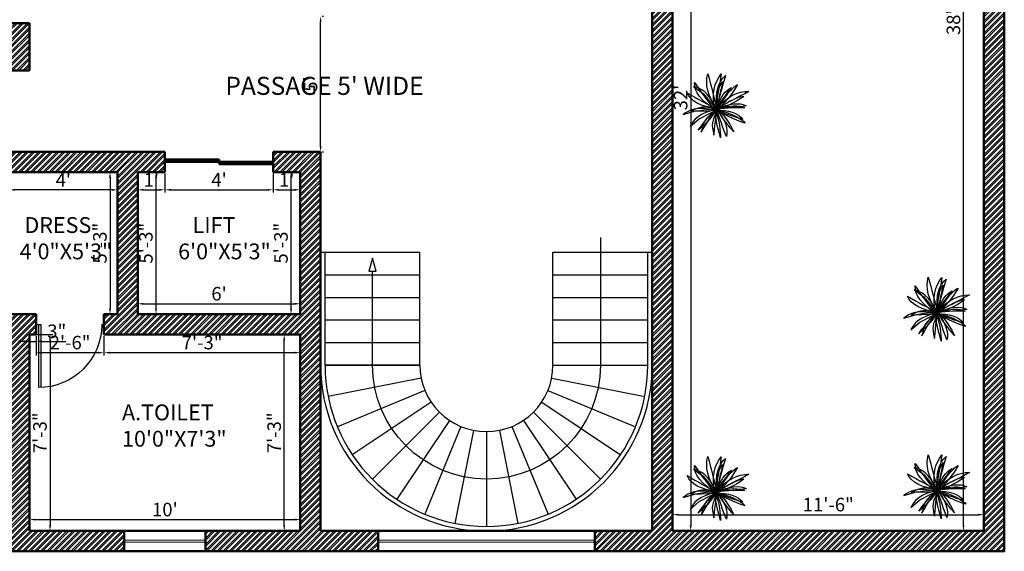
# Model space of a CAD drawing. Units: inches. Extents: x 3590 to 5167, y 65 to 1917.
# Tile 24 of 100: x 4644 to 5080, y 735 to 971. Entities that reach past the tile are written whole.
import ezdxf

# ---------------------------------------------------------------- set-up
doc = ezdxf.new("R2010")
doc.units = ezdxf.units.IN
for name, color, linetype, lineweight in [('A-ANNO-DIMS', 2, 'Continuous', 18), ('A-AREA-IDEN', 7, 'Continuous', 18), ('A-DOOR', 3, 'Continuous', 25), ('A-FLOR-STRS', 7, 'Continuous', 25), ('A-GLAZ', 4, 'Continuous', 18), ('A-WALL', 7, 'Continuous', 50), ('A-WALL-PATT', 251, 'Continuous', 13), ('L-PLNT', 94, 'Continuous', 18)]:
    doc.layers.add(name, color=color, linetype=linetype, lineweight=lineweight)
doc.layers.add('DIENHOA', color=3, linetype='Continuous')
doc.styles.get("Standard").update_dxf_attribs({"font": 'arial.ttf'})
doc.dimstyles.new('ISO-25', dxfattribs={"dimtxt": 9, "dimasz": 2.5, "dimexe": 1.25, "dimexo": 0.625, "dimtad": 1, "dimdec": 1, "dimlunit": 3, "dimtxsty": 'Standard', "dimcen": 2.5, "dimadec": 0, "dimazin": 0, "dimtfac": 1, "dimtdec": 1, "dimtmove": 0, "dimatfit": 3, "dimfxl": 1, "dimarcsym": 0})

# ---------------------------------------------------------------- blocks, each defined once
blk = doc.blocks.new('*U104')
blk.add_line((-21, 0), (21, 0))
blk = doc.blocks.new('*U103')
at = {"layer": 'A-FLOR-STRS', "color": 0, "linetype": 'ByBlock', "lineweight": -2, "transparency": 16777216}
for p, rotation in [((4076.01, 1459), 89.99999999999982), ((4066.16, 1458.03), 101.2499999999998), ((4085.86, 1458.03), 78.7499999999998), ((4056.69, 1455.15), 112.4999999999998), ((4095.34, 1455.15), 67.4999999999998), ((4047.96, 1450.49), 123.7499999999997), ((4104.07, 1450.49), 56.24999999999984), ((4040.3, 1444.21), 134.9999999999996), ((4111.72, 1444.21), 44.99999999999992), ((4034.02, 1436.56), 146.2499999999996), ((4118, 1436.56), 33.74999999999991), ((4029.36, 1427.82), 157.4999999999995), ((4122.67, 1427.82), 22.49999999999996), ((4026.48, 1418.35), 168.7499999999995), ((4125.54, 1418.35), 11.25), ((4025.51, 1408.5), 180)]:
    blk.add_blockref('*U104', p, dxfattribs=dict(at, rotation=rotation))
blk.add_blockref('*U104', (4126.51, 1408.5), dxfattribs=at)
blk = doc.blocks.new('D2')
for p, q in [((1, 0), (1, 28)), ((2, 0), (2, 27.98)), ((0, 0), (2, 0)), ((29, 0), (30, 0))]:
    blk.add_line(p, q)
at = {"ltscale": 0.5}
blk.add_arc((1, 0), 28, 0, 90, dxfattribs=at)
blk = doc.blocks.new('Cay03_mb')
at = {"layer": 'DIENHOA'}
for p, q in [((79, 504), (119, 555)), ((119, 555), (166, 599)), ((166, 599), (142, 519)), ((-365, 390), (-414, 403)), ((-414, 403), (-240, 278)), ((-315, 371), (-365, 390)), ((-264, 343), (-315, 371)), ((10, 295), (25, 374)), ((25, 374), (49, 444)), ((49, 444), (79, 504)), ((97, 366), (76, 291)), ((119, 442), (97, 366)), ((142, 519), (119, 442)), ((-211, 305), (-264, 343)), ((-240, 278), (-88, 95)), ((-158, 252), (-211, 305)), ((-104, 184), (-158, 252)), ((-50, 98), (-104, 184)), ((0, 105), (2, 206)), ((2, 206), (10, 295)), ((56, 216), (37, 142)), ((76, 291), (56, 216)), ((147, 144), (219, 200)), ((219, 200), (291, 243)), ((364, 193), (290, 155)), ((291, 243), (363, 275)), ((363, 275), (437, 297)), ((438, 231), (364, 193)), ((437, 297), (511, 310)), ((512, 271), (438, 231)), ((511, 310), (586, 314)), ((586, 314), (512, 271)), ((-345, 5), (-400, -17)), ((-299, 20), (-345, 5)), ((-255, 27), (-299, 20)), ((-208, 28), (-255, 27)), ((-153, 22), (-208, 28)), ((-83, 10), (-153, 22)), ((-88, 95), (5, -8)), ((5, -8), (-83, 10)), ((5, -8), (-50, 98)), ((5, -8), (0, 105)), ((5, -8), (76, 75)), ((20, 68), (5, -8)), ((75, 36), (5, -8)), ((5, -8), (100, 18)), ((46, 1), (5, -8)), ((37, 142), (20, 68)), ((97, 7), (46, 1)), ((145, 77), (75, 36)), ((76, 75), (147, 144)), ((155, 12), (97, 7)), ((100, 18), (182, 37)), ((217, 117), (145, 77)), ((220, 15), (155, 12)), ((182, 37), (253, 49)), ((290, 155), (217, 117)), ((289, 17), (220, 15)), ((253, 49), (315, 54)), ((362, 19), (289, 17)), ((315, 54), (369, 53)), ((436, 19), (362, 19)), ((369, 53), (419, 47)), ((419, 47), (465, 35)), ((510, 19), (436, 19)), ((465, 35), (510, 19)), ((-400, -17), (-468, -48)), ((-468, -48), (-376, -38)), ((-376, -38), (-295, -28)), ((-295, -28), (-226, -19)), ((-226, -19), (-166, -11)), ((-216, -236), (-166, -174)), ((-166, -11), (-114, -6)), ((-166, -174), (-120, -122)), ((-120, -122), (-80, -80)), ((-75, -127), (-118, -181)), ((-114, -6), (-69, -3)), ((-80, -80), (-45, -46)), ((-33, -69), (-75, -127)), ((-69, -3), (-30, -3)), ((-45, -46), (-17, -22)), ((5, -8), (-33, -69)), ((-30, -3), (5, -8)), ((-17, -22), (5, -8)), ((5, -8), (57, -73)), ((26, -64), (5, -8)), ((5, -8), (113, -40)), ((53, -42), (5, -8)), ((47, -126), (26, -64)), ((69, -191), (47, -126)), ((107, -76), (53, -42)), ((57, -73), (100, -139)), ((100, -139), (136, -204)), ((166, -110), (107, -76)), ((113, -40), (207, -74)), ((229, -143), (166, -110)), ((207, -74), (290, -108)), ((296, -175), (229, -143)), ((290, -108), (359, -141)), ((367, -205), (296, -175)), ((359, -141), (417, -174)), ((417, -174), (463, -204)), ((-330, -387), (-271, -307)), ((-291, -355), (-330, -387)), ((-250, -318), (-291, -355)), ((-271, -307), (-216, -236)), ((-206, -276), (-250, -318)), ((-162, -231), (-206, -276)), ((-118, -181), (-162, -231)), ((91, -257), (69, -191)), ((113, -322), (91, -257)), ((135, -386), (113, -322)), ((136, -204), (163, -268)), ((163, -268), (181, -330)), ((181, -330), (190, -390)), ((442, -233), (367, -205)), ((519, -258), (442, -233)), ((463, -204), (496, -232)), ((496, -232), (519, -258)), ((158, -445), (135, -386)), ((180, -499), (158, -445)), ((190, -446), (180, -499)), ((190, -390), (190, -446))]:
    blk.add_line(p, q, dxfattribs=at)
for points in [[(24, -5), (-41, 82), (-92, 167), (-130, 249), (-156, 330), (-170, 408), (-175, 484), (-170, 559), (-157, 633)], [(-157, 633), (-132, 551), (-111, 470), (-90, 389), (-70, 309), (-49, 229), (-27, 150), (-3, 72), (24, -5)], [(-16, -27), (-38, 80), (-49, 178), (-49, 269), (-39, 353), (-19, 430), (9, 501), (45, 567), (88, 629)], [(88, 629), (75, 544), (61, 461), (46, 379), (31, 298), (16, 217), (3, 136), (-8, 55), (-16, -27)], [(-396, 474), (-348, 406), (-301, 339), (-254, 275), (-208, 212), (-162, 151), (-115, 91), (-66, 32), (-16, -27)], [(-16, -27), (-108, 39), (-187, 102), (-252, 163), (-305, 224), (-345, 285), (-374, 347), (-390, 409), (-396, 474)], [(273, 387), (228, 329), (182, 270), (138, 212), (97, 156), (60, 103), (28, 55), (2, 11), (-16, -27)], [(-16, -27), (21, 64), (57, 140), (91, 203), (125, 255), (160, 297), (195, 332), (233, 362), (273, 387)], [(24, -5), (20, 93), (20, 177), (25, 249), (34, 310), (47, 363), (65, 409), (87, 452), (113, 492)], [(113, 492), (96, 420), (79, 347), (64, 276), (50, 208), (38, 145), (30, 87), (25, 36), (24, -5)], [(384, 437), (342, 368), (298, 302), (253, 239), (206, 181), (159, 127), (113, 78), (68, 34), (24, -5)], [(24, -5), (80, 92), (134, 176), (186, 248), (234, 309), (279, 357), (319, 395), (355, 421), (384, 437)], [(-530, 290), (-458, 248), (-388, 208), (-319, 169), (-251, 131), (-183, 95), (-115, 60), (-46, 26), (24, -5)], [(24, -5), (-87, 15), (-185, 40), (-270, 68), (-344, 101), (-406, 140), (-457, 184), (-499, 233), (-530, 290)], [(497, 224), (429, 178), (362, 137), (294, 99), (227, 66), (162, 37), (100, 11), (40, -10), (-16, -27)], [(-16, -27), (75, 38), (160, 92), (237, 136), (307, 170), (368, 195), (420, 213), (463, 222), (497, 224)], [(-16, -27), (-134, -5), (-235, 5), (-322, 5), (-396, -5), (-459, -22), (-512, -46), (-558, -74), (-598, -105)], [(24, -5), (99, 30), (173, 57), (245, 77), (313, 88), (378, 92), (438, 87), (493, 74), (541, 52)], [(541, 52), (484, 43), (421, 35), (354, 28), (285, 21), (216, 14), (148, 8), (83, 2), (24, -5)], [(-598, -105), (-393, -44), (-155, -37), (-16, -27)], [(-472, -320), (-310, -179), (-98, -73), (24, -5)], [(24, -5), (-92, -35), (-188, -68), (-267, -105), (-330, -145), (-380, -187), (-418, -231), (-448, -275), (-472, -320)], [(-276, -424), (-227, -345), (-186, -276), (-150, -216), (-119, -164), (-91, -120), (-66, -82), (-41, -52), (-16, -27)], [(-16, -27), (-85, -86), (-137, -133), (-176, -173), (-204, -210), (-226, -249), (-243, -295), (-258, -352), (-276, -424)], [(24, -5), (-14, -88), (-41, -153), (-60, -205), (-70, -251), (-73, -295), (-69, -344), (-60, -402), (-45, -475)], [(-45, -475), (-34, -383), (-25, -303), (-18, -233), (-12, -173), (-6, -121), (2, -77), (11, -39), (24, -5)], [(76, -524), (49, -428), (27, -342), (9, -264), (-4, -196), (-12, -138), (-17, -90), (-18, -53), (-16, -27)], [(478, -192), (422, -176), (361, -157), (298, -135), (232, -113), (167, -89), (102, -67), (41, -45), (-16, -27)], [(-16, -27), (67, -27), (146, -33), (219, -45), (286, -63), (346, -87), (398, -117), (443, -152), (478, -192)], [(-16, -27), (8, -95), (29, -163), (44, -231), (56, -296), (65, -359), (71, -419), (74, -474), (76, -524)], [(316, -418), (251, -343), (195, -273), (147, -210), (106, -154), (74, -105), (50, -63), (33, -30), (24, -5)], [(24, -5), (75, -57), (122, -111), (164, -165), (203, -219), (237, -273), (267, -324), (294, -373), (316, -418)]]:
    blk.add_lwpolyline(points, dxfattribs=at)
blk = doc.blocks.new('*D135')
at = {"layer": 'A-ANNO-DIMS', "color": 0, "lineweight": -2, "transparency": 16777216}
for p, q in [((4639.27, 902.72), (4639.27, 894.19)), ((4687.27, 902.72), (4687.27, 894.19)), ((4684.77, 895.44), (4641.77, 895.44))]:
    blk.add_line(p, q, dxfattribs=at)
at = {"layer": 'A-ANNO-DIMS', "color": 0, "transparency": 16777216}
for points in [[(4641.77, 895.86), (4641.77, 895.03), (4639.27, 895.44)], [(4684.77, 895.86), (4684.77, 895.03), (4687.27, 895.44)]]:
    blk.add_solid(points, dxfattribs=at)
at = {"layer": 'Defpoints', "color": 0, "transparency": 16777216}
for p in [(4639.27, 903.35), (4687.27, 903.35), (4639.27, 895.44)]:
    blk.add_point(p, dxfattribs=at)
at = {"layer": 'A-ANNO-DIMS', "color": 0, "transparency": 16777216, "insert": (4663.27, 899.07), "char_height": 6, "attachment_point": 5}
blk.add_mtext("4'", dxfattribs=at)
blk = doc.blocks.new('*D136')
at = {"layer": 'A-ANNO-DIMS', "color": 0, "lineweight": -2, "transparency": 16777216}
for p, q in [((4686.65, 903.35), (4682.7, 903.35)), ((4683.95, 900.85), (4683.95, 842.85)), ((4686.65, 840.35), (4682.7, 840.35))]:
    blk.add_line(p, q, dxfattribs=at)
at = {"layer": 'A-ANNO-DIMS', "color": 0, "transparency": 16777216}
for points in [[(4683.54, 900.85), (4684.37, 900.85), (4683.95, 903.35)], [(4683.54, 842.85), (4684.37, 842.85), (4683.95, 840.35)]]:
    blk.add_solid(points, dxfattribs=at)
at = {"layer": 'Defpoints', "color": 0, "transparency": 16777216}
for p in [(4687.27, 903.35), (4683.95, 840.35), (4687.27, 840.35)]:
    blk.add_point(p, dxfattribs=at)
at = {"layer": 'A-ANNO-DIMS', "color": 0, "transparency": 16777216, "insert": (4680.26, 871.85), "char_height": 6, "attachment_point": 5, "rotation": 90}
blk.add_mtext('5\'-3"', dxfattribs=at)
blk = doc.blocks.new('*D137')
at = {"layer": 'A-ANNO-DIMS', "color": 0, "lineweight": -2, "transparency": 16777216}
for p, q in [((4648.27, 830.72), (4648.27, 827.11)), ((4651.27, 830.72), (4651.27, 827.11)), ((4645.77, 828.36), (4643.27, 828.36)), ((4648.27, 828.36), (4651.27, 828.36)), ((4653.77, 828.36), (4664.42, 828.36))]:
    blk.add_line(p, q, dxfattribs=at)
at = {"layer": 'A-ANNO-DIMS', "color": 0, "transparency": 16777216}
for points in [[(4645.77, 828.78), (4645.77, 827.94), (4648.27, 828.36)], [(4653.77, 828.78), (4653.77, 827.94), (4651.27, 828.36)]]:
    blk.add_solid(points, dxfattribs=at)
at = {"layer": 'Defpoints', "color": 0, "transparency": 16777216}
for p in [(4648.27, 831.35), (4651.27, 831.35), (4651.27, 828.36)]:
    blk.add_point(p, dxfattribs=at)
at = {"layer": 'A-ANNO-DIMS', "color": 0, "transparency": 16777216, "insert": (4660.35, 832.05), "char_height": 6, "attachment_point": 5}
blk.add_mtext('3"', dxfattribs=at)
blk = doc.blocks.new('*D138')
at = {"layer": 'A-ANNO-DIMS', "color": 0, "lineweight": -2, "transparency": 16777216}
for p, q in [((4651.27, 830.72), (4651.27, 822.1)), ((4681.27, 830.72), (4681.27, 822.1)), ((4653.77, 823.35), (4678.77, 823.35))]:
    blk.add_line(p, q, dxfattribs=at)
at = {"layer": 'A-ANNO-DIMS', "color": 0, "transparency": 16777216}
for points in [[(4653.77, 823.76), (4653.77, 822.93), (4651.27, 823.35)], [(4678.77, 823.76), (4678.77, 822.93), (4681.27, 823.35)]]:
    blk.add_solid(points, dxfattribs=at)
at = {"layer": 'Defpoints', "color": 0, "transparency": 16777216}
for p in [(4651.27, 831.35), (4681.27, 831.35), (4681.27, 823.35)]:
    blk.add_point(p, dxfattribs=at)
at = {"layer": 'A-ANNO-DIMS', "color": 0, "transparency": 16777216, "insert": (4666.27, 827.04), "char_height": 6, "attachment_point": 5}
blk.add_mtext('2\'-6"', dxfattribs=at)
blk = doc.blocks.new('*D139')
at = {"layer": 'A-ANNO-DIMS', "color": 0, "lineweight": -2, "transparency": 16777216}
for p, q in [((4681.27, 830.72), (4681.27, 822.1)), ((4768.27, 830.72), (4768.27, 822.1)), ((4683.77, 823.35), (4765.77, 823.35))]:
    blk.add_line(p, q, dxfattribs=at)
at = {"layer": 'A-ANNO-DIMS', "color": 0, "transparency": 16777216}
for points in [[(4683.77, 823.76), (4683.77, 822.93), (4681.27, 823.35)], [(4765.77, 823.76), (4765.77, 822.93), (4768.27, 823.35)]]:
    blk.add_solid(points, dxfattribs=at)
at = {"layer": 'Defpoints', "color": 0, "transparency": 16777216}
for p in [(4681.27, 831.35), (4768.27, 831.35), (4768.27, 823.35)]:
    blk.add_point(p, dxfattribs=at)
at = {"layer": 'A-ANNO-DIMS', "color": 0, "transparency": 16777216, "insert": (4724.77, 827.04), "char_height": 6, "attachment_point": 5}
blk.add_mtext('7\'-3"', dxfattribs=at)
blk = doc.blocks.new('*D140')
at = {"layer": 'A-ANNO-DIMS', "color": 0, "lineweight": -2, "transparency": 16777216}
for p, q in [((4648.9, 831.35), (4658.62, 831.35)), ((4657.37, 828.85), (4657.37, 746.85)), ((4648.9, 744.35), (4658.62, 744.35))]:
    blk.add_line(p, q, dxfattribs=at)
at = {"layer": 'A-ANNO-DIMS', "color": 0, "transparency": 16777216}
for points in [[(4656.95, 828.85), (4657.78, 828.85), (4657.37, 831.35)], [(4656.95, 746.85), (4657.78, 746.85), (4657.37, 744.35)]]:
    blk.add_solid(points, dxfattribs=at)
at = {"layer": 'Defpoints', "color": 0, "transparency": 16777216}
for p in [(4648.27, 831.35), (4648.27, 744.35), (4657.37, 744.35)]:
    blk.add_point(p, dxfattribs=at)
at = {"layer": 'A-ANNO-DIMS', "color": 0, "transparency": 16777216, "insert": (4653.68, 787.85), "char_height": 6, "attachment_point": 5, "rotation": 90}
blk.add_mtext('7\'-3"', dxfattribs=at)
blk = doc.blocks.new('*D141')
at = {"layer": 'A-ANNO-DIMS', "color": 0, "lineweight": -2, "transparency": 16777216}
for p, q in [((4648.27, 744.97), (4648.27, 750.64)), ((4768.27, 744.97), (4768.27, 750.64)), ((4650.77, 749.39), (4765.77, 749.39))]:
    blk.add_line(p, q, dxfattribs=at)
at = {"layer": 'A-ANNO-DIMS', "color": 0, "transparency": 16777216}
for points in [[(4650.77, 749.8), (4650.77, 748.97), (4648.27, 749.39)], [(4765.77, 749.8), (4765.77, 748.97), (4768.27, 749.39)]]:
    blk.add_solid(points, dxfattribs=at)
at = {"layer": 'Defpoints', "color": 0, "transparency": 16777216}
for p in [(4768.27, 749.39), (4648.27, 744.35), (4768.27, 744.35)]:
    blk.add_point(p, dxfattribs=at)
at = {"layer": 'A-ANNO-DIMS', "color": 0, "transparency": 16777216, "insert": (4708.27, 753.08), "char_height": 6, "attachment_point": 5}
blk.add_mtext("10'", dxfattribs=at)
blk = doc.blocks.new('*D142')
at = {"layer": 'A-ANNO-DIMS', "color": 0, "lineweight": -2, "transparency": 16777216}
for p, q in [((4767.65, 831.35), (4759.91, 831.35)), ((4761.16, 746.85), (4761.16, 828.85)), ((4767.65, 744.35), (4759.91, 744.35))]:
    blk.add_line(p, q, dxfattribs=at)
at = {"layer": 'A-ANNO-DIMS', "color": 0, "transparency": 16777216}
for points in [[(4760.74, 828.85), (4761.57, 828.85), (4761.16, 831.35)], [(4760.74, 746.85), (4761.57, 746.85), (4761.16, 744.35)]]:
    blk.add_solid(points, dxfattribs=at)
at = {"layer": 'Defpoints', "color": 0, "transparency": 16777216}
for p in [(4761.16, 831.35), (4768.27, 831.35), (4768.27, 744.35)]:
    blk.add_point(p, dxfattribs=at)
at = {"layer": 'A-ANNO-DIMS', "color": 0, "transparency": 16777216, "insert": (4757.47, 787.85), "char_height": 6, "attachment_point": 5, "rotation": 90}
blk.add_mtext('7\'-3"', dxfattribs=at)
blk = doc.blocks.new('*D143')
at = {"layer": 'A-ANNO-DIMS', "color": 0, "lineweight": -2, "transparency": 16777216}
for p, q in [((4696.9, 903.35), (4705.58, 903.35)), ((4704.33, 900.85), (4704.33, 842.85)), ((4696.9, 840.35), (4705.58, 840.35))]:
    blk.add_line(p, q, dxfattribs=at)
at = {"layer": 'A-ANNO-DIMS', "color": 0, "transparency": 16777216}
for points in [[(4703.91, 900.85), (4704.74, 900.85), (4704.33, 903.35)], [(4703.91, 842.85), (4704.74, 842.85), (4704.33, 840.35)]]:
    blk.add_solid(points, dxfattribs=at)
at = {"layer": 'Defpoints', "color": 0, "transparency": 16777216}
for p in [(4696.27, 903.35), (4696.27, 840.35), (4704.33, 840.35)]:
    blk.add_point(p, dxfattribs=at)
at = {"layer": 'A-ANNO-DIMS', "color": 0, "transparency": 16777216, "insert": (4700.63, 871.85), "char_height": 6, "attachment_point": 5, "rotation": 90}
blk.add_mtext('5\'-3"', dxfattribs=at)
blk = doc.blocks.new('*D144')
at = {"layer": 'A-ANNO-DIMS', "color": 0, "lineweight": -2, "transparency": 16777216}
for p, q in [((4696.27, 840.97), (4696.27, 846.24)), ((4698.77, 844.99), (4765.77, 844.99)), ((4768.27, 840.97), (4768.27, 846.24))]:
    blk.add_line(p, q, dxfattribs=at)
at = {"layer": 'A-ANNO-DIMS', "color": 0, "transparency": 16777216}
for points in [[(4698.77, 845.41), (4698.77, 844.57), (4696.27, 844.99)], [(4765.77, 845.41), (4765.77, 844.57), (4768.27, 844.99)]]:
    blk.add_solid(points, dxfattribs=at)
at = {"layer": 'Defpoints', "color": 0, "transparency": 16777216}
for p in [(4768.27, 844.99), (4696.27, 840.35), (4768.27, 840.35)]:
    blk.add_point(p, dxfattribs=at)
at = {"layer": 'A-ANNO-DIMS', "color": 0, "transparency": 16777216, "insert": (4732.27, 848.68), "char_height": 6, "attachment_point": 5}
blk.add_mtext("6'", dxfattribs=at)
blk = doc.blocks.new('*D145')
at = {"layer": 'A-ANNO-DIMS', "color": 0, "lineweight": -2, "transparency": 16777216}
for p, q in [((4767.65, 903.35), (4762.93, 903.35)), ((4764.18, 842.85), (4764.18, 900.85)), ((4767.65, 840.35), (4762.93, 840.35))]:
    blk.add_line(p, q, dxfattribs=at)
at = {"layer": 'A-ANNO-DIMS', "color": 0, "transparency": 16777216}
for points in [[(4763.77, 900.85), (4764.6, 900.85), (4764.18, 903.35)], [(4763.77, 842.85), (4764.6, 842.85), (4764.18, 840.35)]]:
    blk.add_solid(points, dxfattribs=at)
at = {"layer": 'Defpoints', "color": 0, "transparency": 16777216}
for p in [(4764.18, 903.35), (4768.27, 903.35), (4768.27, 840.35)]:
    blk.add_point(p, dxfattribs=at)
at = {"layer": 'A-ANNO-DIMS', "color": 0, "transparency": 16777216, "insert": (4760.49, 871.85), "char_height": 6, "attachment_point": 5, "rotation": 90}
blk.add_mtext('5\'-3"', dxfattribs=at)
blk = doc.blocks.new('*D146')
at = {"layer": 'A-ANNO-DIMS', "color": 0, "lineweight": -2, "transparency": 16777216}
for p, q in [((4696.27, 902.72), (4696.27, 894.24)), ((4708.27, 902.72), (4708.27, 894.24)), ((4698.77, 895.49), (4705.77, 895.49))]:
    blk.add_line(p, q, dxfattribs=at)
at = {"layer": 'A-ANNO-DIMS', "color": 0, "transparency": 16777216}
for points in [[(4698.77, 895.91), (4698.77, 895.08), (4696.27, 895.49)], [(4705.77, 895.91), (4705.77, 895.08), (4708.27, 895.49)]]:
    blk.add_solid(points, dxfattribs=at)
at = {"layer": 'Defpoints', "color": 0, "transparency": 16777216}
for p in [(4696.27, 903.35), (4708.27, 903.35), (4708.27, 895.49)]:
    blk.add_point(p, dxfattribs=at)
at = {"layer": 'A-ANNO-DIMS', "color": 0, "transparency": 16777216, "insert": (4702.27, 899.13), "char_height": 6, "attachment_point": 5}
blk.add_mtext("1'", dxfattribs=at)
blk = doc.blocks.new('*D147')
at = {"layer": 'A-ANNO-DIMS', "color": 0, "lineweight": -2, "transparency": 16777216}
for p, q in [((4708.27, 902.72), (4708.27, 894.24)), ((4756.27, 902.72), (4756.27, 894.24)), ((4710.77, 895.49), (4753.77, 895.49))]:
    blk.add_line(p, q, dxfattribs=at)
at = {"layer": 'A-ANNO-DIMS', "color": 0, "transparency": 16777216}
for points in [[(4710.77, 895.91), (4710.77, 895.08), (4708.27, 895.49)], [(4753.77, 895.91), (4753.77, 895.08), (4756.27, 895.49)]]:
    blk.add_solid(points, dxfattribs=at)
at = {"layer": 'Defpoints', "color": 0, "transparency": 16777216}
for p in [(4708.27, 903.35), (4756.27, 903.35), (4756.27, 895.49)]:
    blk.add_point(p, dxfattribs=at)
at = {"layer": 'A-ANNO-DIMS', "color": 0, "transparency": 16777216, "insert": (4732.27, 899.12), "char_height": 6, "attachment_point": 5}
blk.add_mtext("4'", dxfattribs=at)
blk = doc.blocks.new('*D148')
at = {"layer": 'A-ANNO-DIMS', "color": 0, "lineweight": -2, "transparency": 16777216}
for p, q in [((4756.27, 902.72), (4756.27, 894.24)), ((4768.27, 902.72), (4768.27, 894.24)), ((4758.77, 895.49), (4765.77, 895.49))]:
    blk.add_line(p, q, dxfattribs=at)
at = {"layer": 'A-ANNO-DIMS', "color": 0, "transparency": 16777216}
for points in [[(4758.77, 895.91), (4758.77, 895.08), (4756.27, 895.49)], [(4765.77, 895.91), (4765.77, 895.08), (4768.27, 895.49)]]:
    blk.add_solid(points, dxfattribs=at)
at = {"layer": 'Defpoints', "color": 0, "transparency": 16777216}
for p in [(4756.27, 903.35), (4768.27, 903.35), (4768.27, 895.49)]:
    blk.add_point(p, dxfattribs=at)
at = {"layer": 'A-ANNO-DIMS', "color": 0, "transparency": 16777216, "insert": (4762.27, 899.13), "char_height": 6, "attachment_point": 5}
blk.add_mtext("1'", dxfattribs=at)
blk = doc.blocks.new('*D149')
at = {"layer": 'A-ANNO-DIMS', "color": 0, "lineweight": -2, "transparency": 16777216}
for p, q in [((4933.27, 744.97), (4933.27, 752.82)), ((4935.77, 751.57), (5068.77, 751.57)), ((5071.27, 744.97), (5071.27, 752.82))]:
    blk.add_line(p, q, dxfattribs=at)
at = {"layer": 'A-ANNO-DIMS', "color": 0, "transparency": 16777216}
for points in [[(4935.77, 751.99), (4935.77, 751.16), (4933.27, 751.57)], [(5068.77, 751.99), (5068.77, 751.16), (5071.27, 751.57)]]:
    blk.add_solid(points, dxfattribs=at)
at = {"layer": 'Defpoints', "color": 0, "transparency": 16777216}
for p in [(5071.27, 751.57), (4933.27, 744.35), (5071.27, 744.35)]:
    blk.add_point(p, dxfattribs=at)
at = {"layer": 'A-ANNO-DIMS', "color": 0, "transparency": 16777216, "insert": (5002.27, 755.26), "char_height": 6, "attachment_point": 5}
blk.add_mtext('11\'-6"', dxfattribs=at)
blk = doc.blocks.new('*D150')
at = {"layer": 'A-ANNO-DIMS', "color": 0, "lineweight": -2, "transparency": 16777216}
for p, q in [((5070.65, 1206.35), (5060.93, 1206.35)), ((5062.18, 746.85), (5062.18, 1203.85)), ((5070.65, 744.35), (5060.93, 744.35))]:
    blk.add_line(p, q, dxfattribs=at)
at = {"layer": 'A-ANNO-DIMS', "color": 0, "transparency": 16777216}
for points in [[(5061.77, 1203.85), (5062.6, 1203.85), (5062.18, 1206.35)], [(5061.77, 746.85), (5062.6, 746.85), (5062.18, 744.35)]]:
    blk.add_solid(points, dxfattribs=at)
at = {"layer": 'Defpoints', "color": 0, "transparency": 16777216}
for p in [(5062.18, 1206.35), (5071.27, 1206.35), (5071.27, 744.35)]:
    blk.add_point(p, dxfattribs=at)
at = {"layer": 'A-ANNO-DIMS', "color": 0, "transparency": 16777216, "insert": (5058.49, 975.35), "char_height": 6, "attachment_point": 5, "rotation": 90}
blk.add_mtext('38\'-6"', dxfattribs=at)
blk = doc.blocks.new('*D154')
at = {"layer": 'A-ANNO-DIMS', "color": 0, "lineweight": -2, "transparency": 16777216}
for p, q in [((4933.9, 1128.35), (4942.54, 1128.35)), ((4941.29, 1125.85), (4941.29, 746.85)), ((4933.9, 744.35), (4942.54, 744.35))]:
    blk.add_line(p, q, dxfattribs=at)
at = {"layer": 'A-ANNO-DIMS', "color": 0, "transparency": 16777216}
for points in [[(4940.87, 1125.85), (4941.71, 1125.85), (4941.29, 1128.35)], [(4940.87, 746.85), (4941.71, 746.85), (4941.29, 744.35)]]:
    blk.add_solid(points, dxfattribs=at)
at = {"layer": 'Defpoints', "color": 0, "transparency": 16777216}
for p in [(4933.27, 1128.35), (4933.27, 744.35), (4941.29, 744.35)]:
    blk.add_point(p, dxfattribs=at)
at = {"layer": 'A-ANNO-DIMS', "color": 0, "transparency": 16777216, "insert": (4937.6, 936.35), "char_height": 6, "attachment_point": 5, "rotation": 90}
blk.add_mtext("32'", dxfattribs=at)
blk = doc.blocks.new('*D158')
at = {"layer": 'A-ANNO-DIMS', "color": 0, "lineweight": -2, "transparency": 16777216}
for p, q in [((4777.27, 914.85), (4777.27, 969.85)), ((4777.9, 972.35), (4778.52, 972.35)), ((4777.9, 912.35), (4778.52, 912.35))]:
    blk.add_line(p, q, dxfattribs=at)
at = {"layer": 'A-ANNO-DIMS', "color": 0, "transparency": 16777216}
for points in [[(4776.86, 969.85), (4777.69, 969.85), (4777.27, 972.35)], [(4776.86, 914.85), (4777.69, 914.85), (4777.27, 912.35)]]:
    blk.add_solid(points, dxfattribs=at)
at = {"layer": 'Defpoints', "color": 0, "transparency": 16777216}
for p in [(4777.27, 972.35), (4777.27, 972.35), (4777.27, 912.35)]:
    blk.add_point(p, dxfattribs=at)
at = {"layer": 'A-ANNO-DIMS', "color": 0, "transparency": 16777216, "insert": (4773.6, 942.35), "char_height": 6, "attachment_point": 5, "rotation": 90}
blk.add_mtext("5'", dxfattribs=at)

msp = doc.modelspace()

# ---------------------------------------------------------------- hatches: boundary and pattern name
at = {"layer": 'A-WALL-PATT', "transparency": 33554687}
h = msp.add_hatch(dxfattribs=at)
h.set_pattern_fill('ANSI32', color=256, scale=0.2)
h.set_pattern_definition([(45, (0, -590.6538), (-1.3470384, 1.3470384), []), (45, (0.898, -590.6538), (-1.3470384, 1.3470384), [])])
h.paths.add_polyline_path([(4684.27, 1215.35), (4591.27, 1215.35), (4591.27, 1206.35), (4639.27, 1206.35), (4639.27, 1200.35), (4648.27, 1200.35), (4648.27, 1206.35), (4684.27, 1206.35)])
h.paths.add_polyline_path([(4543.27, 1215.35), (4420.27, 1215.35), (4420.27, 1194.35), (4429.27, 1194.35), (4429.27, 1206.35), (4445.92, 1206.35), (4543.27, 1206.35)])
h.paths.add_polyline_path([(4828.27, 1215.35), (4744.27, 1215.35), (4744.27, 1206.35), (4828.27, 1206.35)])
h.paths.add_polyline_path([(4648.27, 1164.35), (4639.27, 1164.35), (4639.27, 1065.35), (4546.27, 1065.35), (4546.27, 1059.35), (4549.27, 1059.35), (4549.27, 963.35), (4429.27, 963.35), (4429.27, 993.35), (4420.27, 993.35), (4420.27, 948.35), (4429.27, 948.35), (4429.27, 954.35), (4639.27, 954.35), (4639.27, 948.35), (4648.27, 948.35), (4648.27, 969.35), (4639.27, 969.35), (4639.27, 963.35), (4555.27, 963.35), (4555.27, 1059.35), (4639.27, 1059.35), (4639.27, 999.35), (4648.27, 999.35)])
h.paths.add_polyline_path([(4516.27, 1065.35), (4429.27, 1065.35), (4429.27, 1146.35), (4420.27, 1146.35), (4420.27, 1029.35), (4429.27, 1029.35), (4429.27, 1059.35), (4516.27, 1059.35)], flags=17)
h.paths.add_polyline_path([(5080.27, 1215.35), (4888.27, 1215.35), (4888.27, 1206.35), (4924.27, 1206.35), (4924.27, 1164.35), (4933.27, 1164.35), (4933.27, 1206.35), (5071.27, 1206.35), (5071.27, 744.35), (4933.27, 744.35), (4933.27, 975.35), (4924.27, 975.35), (4924.27, 744.35), (4898.77, 744.35), (4898.77, 735.35), (5080.27, 735.35)])
h.paths.add_polyline_path([(4933.27, 1128.35), (4924.27, 1128.35), (4924.27, 1047.35), (4933.27, 1047.35)], flags=17)
h.paths.add_polyline_path([(4802.77, 744.35), (4777.27, 744.35), (4777.27, 912.35), (4756.27, 912.35), (4756.27, 903.35), (4768.27, 903.35), (4768.27, 840.35), (4696.27, 840.35), (4696.27, 903.35), (4708.27, 903.35), (4708.27, 912.35), (4639.27, 912.35), (4639.27, 903.35), (4687.27, 903.35), (4687.27, 840.35), (4681.27, 840.35), (4681.27, 831.35), (4768.27, 831.35), (4768.27, 744.35), (4726.27, 744.35), (4726.27, 735.35), (4802.77, 735.35)])
h.paths.add_polyline_path([(4690.27, 744.35), (4648.27, 744.35), (4648.27, 762.21), (4648.27, 831.35), (4651.27, 831.35), (4651.27, 840.35), (4639.27, 840.35), (4639.27, 744.35), (4633.27, 744.35), (4633.27, 735.35), (4690.27, 735.35)])
h.paths.add_polyline_path([(4585.27, 744.35), (4584.72, 744.35), (4429.27, 744.35), (4429.27, 900.35), (4420.27, 900.35), (4420.27, 735.35), (4585.27, 735.35)])

# ---------------------------------------------------------------- linework, layer by layer
at = {"layer": 'A-FLOR-STRS'}
for p, q in [((4777.27, 867.85), (4821.27, 867.85)), ((4779.27, 817.85), (4779.27, 867.85)), ((4821.27, 817.85), (4821.27, 867.85)), ((4880.27, 867.85), (4924.27, 867.85)), ((4880.27, 817.85), (4880.27, 867.85)), ((4922.27, 817.85), (4922.27, 867.85)), ((4779.27, 857.85), (4821.27, 857.85)), ((4880.27, 857.85), (4922.27, 857.85)), ((4779.27, 847.85), (4821.27, 847.85)), ((4880.27, 847.85), (4922.27, 847.85)), ((4779.27, 837.85), (4821.27, 837.85)), ((4880.27, 837.85), (4922.27, 837.85)), ((4779.27, 827.85), (4821.27, 827.85)), ((4880.27, 827.85), (4922.27, 827.85)), ((4779.27, 817.85), (4821.27, 817.85))]:
    msp.add_line(p, q, dxfattribs=at)
msp.add_lwpolyline([(4901.27, 874.29), (4901.27, 817.85, -1), (4800.27, 817.85), (4800.27, 859.46)], format="xyb", dxfattribs=at)
msp.add_lwpolyline([(4800.27, 865.22), (4798.64, 859.46), (4801.91, 859.46)], close=True, dxfattribs=at)
for radius in [73.5, 71.5, 29.5]:
    msp.add_arc((4850.77, 817.85), radius, 180, 0, dxfattribs=at)
at = {"layer": 'A-GLAZ'}
for p, q in [((4726.27, 740.35), (4690.27, 740.35)), ((4726.27, 739.35), (4690.27, 739.35)), ((4898.77, 740.35), (4802.77, 740.35)), ((4898.77, 739.35), (4802.77, 739.35))]:
    msp.add_line(p, q, dxfattribs=at)
at = {"layer": 'A-WALL'}
for p, q in [((5071.27, 744.35), (5071.27, 1206.35)), ((4924.27, 744.35), (4924.27, 1128.35)), ((4933.27, 744.35), (4933.27, 1128.35)), ((4648.27, 969.35), (4639.27, 969.35)), ((4648.27, 948.35), (4648.27, 969.35)), ((4648.27, 948.35), (4639.27, 948.35)), ((4708.27, 912.35), (4639.27, 912.35)), ((4708.27, 903.35), (4708.27, 912.35)), ((4777.27, 912.35), (4756.27, 912.35)), ((4756.27, 903.35), (4756.27, 912.35)), ((4777.27, 744.35), (4777.27, 912.35)), ((4708.27, 908.85), (4732.27, 908.85)), ((4708.27, 907.85), (4756.27, 907.85)), ((4732.27, 908.85), (4732.27, 906.85)), ((4687.27, 903.35), (4639.27, 903.35)), ((4687.27, 840.35), (4687.27, 903.35)), ((4708.27, 903.35), (4696.27, 903.35)), ((4696.27, 840.35), (4696.27, 903.35)), ((4732.27, 906.85), (4756.27, 906.85)), ((4768.27, 903.35), (4756.27, 903.35)), ((4768.27, 840.35), (4768.27, 903.35)), ((4651.27, 840.35), (4639.27, 840.35)), ((4651.27, 831.35), (4651.27, 840.35)), ((4687.27, 840.35), (4681.27, 840.35)), ((4681.27, 831.35), (4681.27, 840.35)), ((4768.27, 840.35), (4696.27, 840.35)), ((4651.27, 831.35), (4648.27, 831.35)), ((4648.27, 744.35), (4648.27, 831.35)), ((4768.27, 831.35), (4681.27, 831.35)), ((4768.27, 744.35), (4768.27, 831.35)), ((4768.27, 744.35), (4648.27, 744.35)), ((4690.27, 744.35), (4690.27, 735.35)), ((4726.27, 744.35), (4726.27, 735.35)), ((4924.27, 744.35), (4777.27, 744.35)), ((4802.77, 744.35), (4802.77, 735.35)), ((4898.77, 744.35), (4898.77, 735.35)), ((5071.27, 744.35), (4933.27, 744.35))]:
    msp.add_line(p, q, dxfattribs=at)
msp.add_lwpolyline([(5080.27, 1215.35), (5080.27, 735.35), (4420.27, 735.35), (4420.27, 1215.35)], close=True, dxfattribs=at)

# ---------------------------------------------------------------- block references
at = {"layer": 'A-DOOR', "xscale": -1, "rotation": 180}
msp.add_blockref('D2', (4651.27, 835.85), dxfattribs=at)
at = {"layer": 'A-FLOR-STRS', "xscale": -1, "rotation": 180}
msp.add_blockref('*U103', (774.76, 2226.34), dxfattribs=at)
at = {"layer": 'L-PLNT', "xscale": 0.0245452446402784, "yscale": 0.0245452446402784, "zscale": 0.0245452446402784}
for p in [(4952.67, 931.38), (5050.43, 841.24), (4952.67, 761.79), (5050.43, 762.59)]:
    msp.add_blockref('Cay03_mb', p, dxfattribs=at)

# ---------------------------------------------------------------- texts
at = {"layer": 'A-AREA-IDEN', "attachment_point": 1}
for s, width, insert, char_height in [("{\\fTimes New Roman|b0|i0|c0|p18;PASSAGE 5' WIDE}", 131.4857, (4735.07, 945.54), 8), ('{\\fTimes New Roman|b0|i0|c0|p18; DRESS\\P4\'0"X5\'3"}', 67.3508, (4643.89, 883.37), 7), ('{\\fTimes New Roman|b0|i0|c0|p18;   LIFT\\P6\'0"X5\'3"}', 67.3508, (4714.15, 883.37), 7), ('{\\fTimes New Roman|b0|i0|c0|p18;A.TOILET\\P10\'0"X7\'3"}', 67.3508, (4689.28, 800.38), 7)]:
    msp.add_mtext_dynamic_manual_height_columns(s, width=width, gutter_width=12.5, heights=[0], dxfattribs=dict(at, insert=insert, char_height=char_height))

# ---------------------------------------------------------------- dimensions: what is measured, and where the dimension line sits
at = {"layer": 'A-ANNO-DIMS'}
for base, p1, p2, override, picture, middle in [((5062.18, 1206.35), (5071.27, 744.35), (5071.27, 1206.35), {"dimtxt": 6, "dimclrd": 0, "dimclre": 0, "dimclrt": 0}, '*D150', (5058.49, 975.35)), ((4941.29, 744.35), (4933.27, 1128.35), (4933.27, 744.35), {"dimtxt": 6, "dimclrd": 0, "dimclre": 0, "dimclrt": 0, "dimtmove": 1}, '*D154', (4937.6, 936.35)), ((4777.27, 972.35), (4777.27, 912.35), (4777.27, 972.35), {"dimtxt": 6, "dimclrd": 0, "dimclre": 0, "dimclrt": 0}, '*D158', (4773.6, 942.35)), ((4683.95, 840.35), (4687.27, 903.35), (4687.27, 840.35), {"dimtxt": 6, "dimclrd": 0, "dimclre": 0, "dimclrt": 0}, '*D136', (4680.26, 871.85)), ((4704.33, 840.35), (4696.27, 903.35), (4696.27, 840.35), {"dimtxt": 6, "dimclrd": 0, "dimclre": 0, "dimclrt": 0}, '*D143', (4700.63, 871.85)), ((4764.18, 903.35), (4768.27, 840.35), (4768.27, 903.35), {"dimtxt": 6, "dimclrd": 0, "dimclre": 0, "dimclrt": 0}, '*D145', (4760.49, 871.85)), ((4657.37, 744.35), (4648.27, 831.35), (4648.27, 744.35), {"dimtxt": 6, "dimclrd": 0, "dimclre": 0, "dimclrt": 0}, '*D140', (4653.68, 787.85)), ((4761.16, 831.35), (4768.27, 744.35), (4768.27, 831.35), {"dimtxt": 6, "dimclrd": 0, "dimclre": 0, "dimclrt": 0}, '*D142', (4757.47, 787.85))]:
    dim = msp.add_linear_dim(base=base, p1=p1, p2=p2, angle=90, dimstyle='ISO-25', override=override, dxfattribs=at)
    dim.commit()
    dim.dimension.update_dxf_attribs({"geometry": picture, "text_midpoint": middle})
for base, p1, p2, override, picture, middle in [((4639.27, 895.44), (4687.27, 903.35), (4639.27, 903.35), {"dimtxt": 6, "dimclrd": 0, "dimclre": 0, "dimclrt": 0}, '*D135', (4663.27, 899.07)), ((4708.27, 895.49), (4696.27, 903.35), (4708.27, 903.35), {"dimtxt": 6, "dimclrd": 0, "dimclre": 0, "dimclrt": 0}, '*D146', (4702.27, 899.13)), ((4756.27, 895.49), (4708.27, 903.35), (4756.27, 903.35), {"dimtxt": 6, "dimclrd": 0, "dimclre": 0, "dimclrt": 0, "dimtmove": 1}, '*D147', (4732.27, 899.12)), ((4768.27, 895.49), (4756.27, 903.35), (4768.27, 903.35), {"dimtxt": 6, "dimclrd": 0, "dimclre": 0, "dimclrt": 0, "dimtmove": 1}, '*D148', (4762.27, 899.13)), ((4768.27, 844.99), (4696.27, 840.35), (4768.27, 840.35), {"dimtxt": 6, "dimclrd": 0, "dimclre": 0, "dimclrt": 0}, '*D144', (4732.27, 848.68)), ((4651.27, 828.36), (4648.27, 831.35), (4651.27, 831.35), {"dimtxt": 6, "dimclrd": 0, "dimclre": 0, "dimclrt": 0}, '*D137', (4660.35, 832.05)), ((4681.27, 823.35), (4651.27, 831.35), (4681.27, 831.35), {"dimtxt": 6, "dimclrd": 0, "dimclre": 0, "dimclrt": 0, "dimtmove": 1}, '*D138', (4666.27, 827.04)), ((4768.27, 823.35), (4681.27, 831.35), (4768.27, 831.35), {"dimtxt": 6, "dimclrd": 0, "dimclre": 0, "dimclrt": 0, "dimtmove": 1}, '*D139', (4724.77, 827.04)), ((5071.27, 751.57), (4933.27, 744.35), (5071.27, 744.35), {"dimtxt": 6, "dimclrd": 0, "dimclre": 0, "dimclrt": 0}, '*D149', (5002.27, 755.26)), ((4768.27, 749.39), (4648.27, 744.35), (4768.27, 744.35), {"dimtxt": 6, "dimclrd": 0, "dimclre": 0, "dimclrt": 0}, '*D141', (4708.27, 753.08))]:
    dim = msp.add_linear_dim(base=base, p1=p1, p2=p2, dimstyle='ISO-25', override=override, dxfattribs=at)
    dim.commit()
    dim.dimension.update_dxf_attribs({"geometry": picture, "text_midpoint": middle})

doc.saveas('drawing.dxf')
